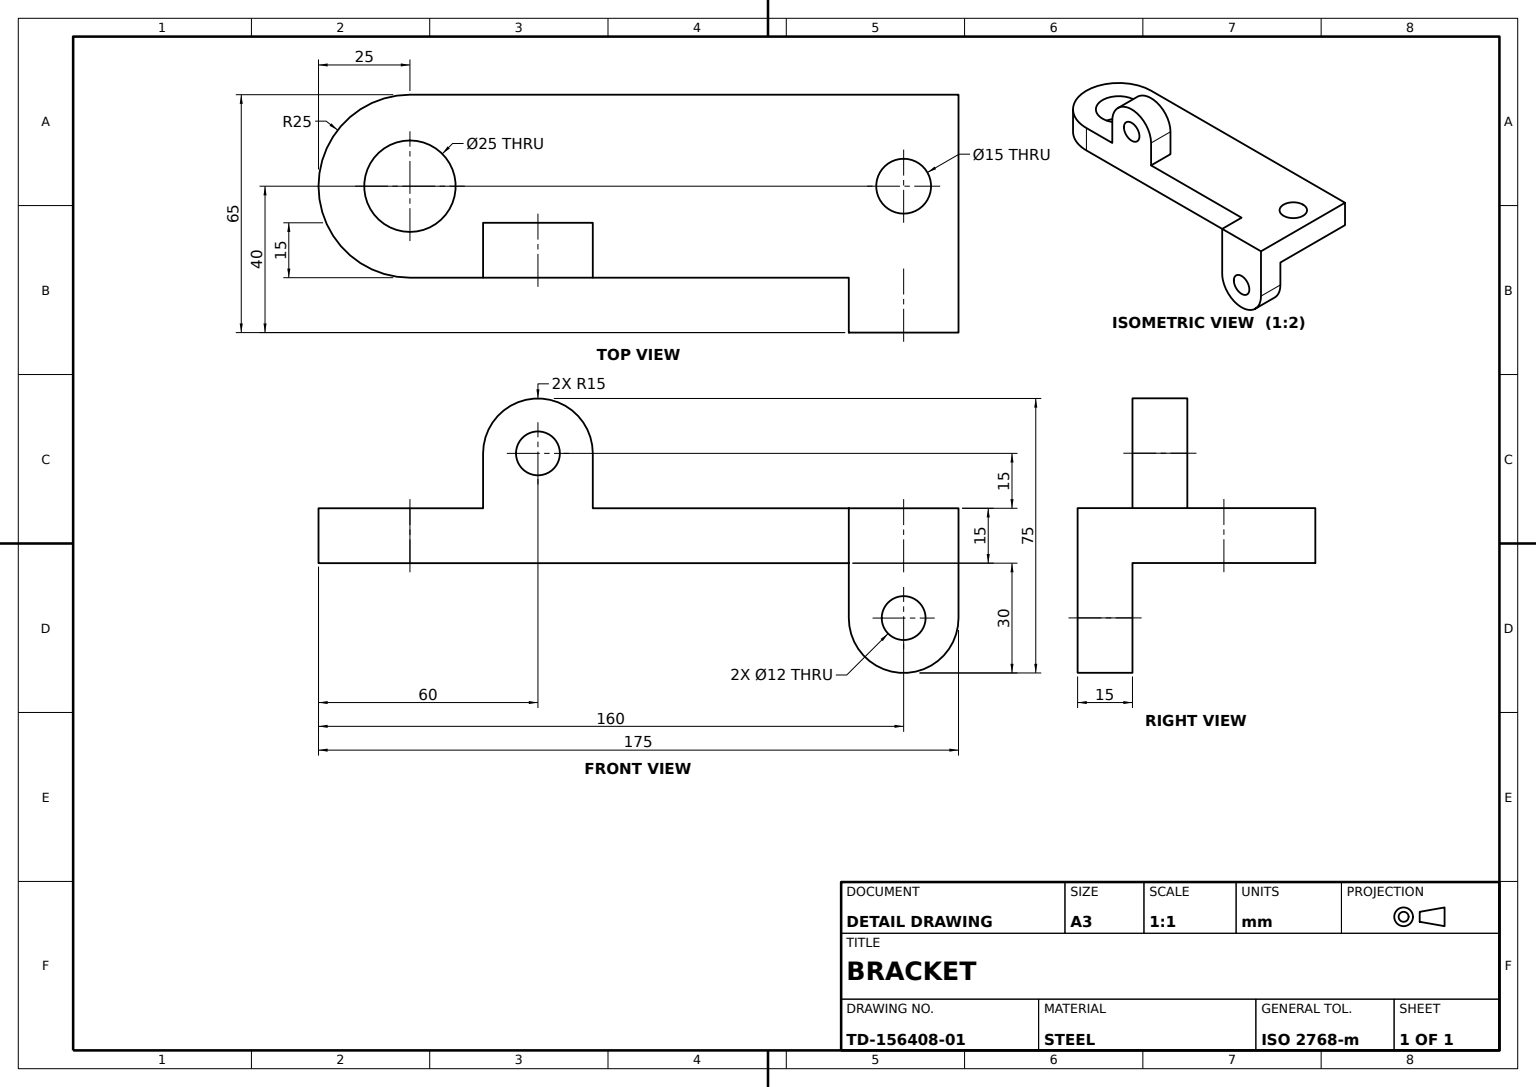
from build123d import *

# Parameters (mm, degrees)
BASE_PROFILE_SKETCH_R       = 12.5
BASE_PROFILE_SKETCH_R_2     = 7.5
BASE_PLATE_DEPTH            = 15
SKETCH1_3_W                 = 30
SKETCH1_3_H                 = 15
LOWER_LUG_DEPTH             = 45
LOWER_LUG_CUT_SKETCH_R      = 6
LOWER_LUG_PROFILE_CUT_DEPTH = 45
UPRIGHT_LUG_SKETCH_R        = 6
UPRIGHT_LUG_12_HOLE_DEPTH   = 15


with BuildPart() as part:
    # Base Profile Sketch → Base Plate (new body)
    with BuildSketch(Plane(origin=(0, 0, 0), x_dir=(1, 0, 0), z_dir=(0, 1, 0))):
        with BuildLine():
            Line((150, 25), (0, 25))
            ThreePointArc((0, 25), (-25, 0), (0, -25))
            Line((0, -25), (102.111825559, -25))
            Line((102.111825559, -25), (120, -25))
            Line((120, -25), (150, -25))
            Line((150, -25), (150, 25))
        make_face()
        with Locations(Location((0, 0, 0), (0, 0, 270))):
            Circle(BASE_PROFILE_SKETCH_R, mode=Mode.SUBTRACT)
        with Locations(Location((135, 0, 0), (0, 0, 270))):
            Circle(BASE_PROFILE_SKETCH_R_2, mode=Mode.SUBTRACT)
    extrude(amount=-BASE_PLATE_DEPTH)

    # Sketch1_3 → Lower Lug (add)
    with BuildSketch(Plane(origin=(0, 0, 0), x_dir=(1, 0, 0), z_dir=(0, 1, 0))):
        with Locations((135, -32.5)):
            Rectangle(SKETCH1_3_W, SKETCH1_3_H)
    extrude(amount=-LOWER_LUG_DEPTH)

    # Lower Lug Cut Sketch → Lower Lug Profile Cut (cut)
    with BuildSketch(Plane.XY.offset(40)):
        with Locations((135, -30)):
            Circle(LOWER_LUG_CUT_SKETCH_R)
        with BuildLine():
            Line((120, -54.887951231), (153.351111221, -54.269822589))
            Line((153.351111221, -54.269822589), (153.351111221, -31.584501417))
            Line((153.351111221, -31.584501417), (150, -30))
            ThreePointArc((150, -30), (135, -45), (120, -30))
            Line((120, -30), (109.958480534, -30))
            Line((109.958480534, -30), (120, -54.887951231))
        make_face()
    extrude(amount=-LOWER_LUG_PROFILE_CUT_DEPTH, mode=Mode.SUBTRACT)

    # Upright Lug Sketch → Upright Lug _12 Hole (add)
    with BuildSketch(Plane.XY.offset(25)):
        with BuildLine():
            Line((20, 15), (20, -3.361922894))
            Line((20, -3.361922894), (50, -3.361922894))
            Line((50, -3.361922894), (50, 15))
            ThreePointArc((50, 15), (35, 30), (20, 15))
        make_face()
        with Locations((35, 15)):
            Circle(UPRIGHT_LUG_SKETCH_R, mode=Mode.SUBTRACT)
    extrude(amount=-UPRIGHT_LUG_12_HOLE_DEPTH)


solid = part.part
